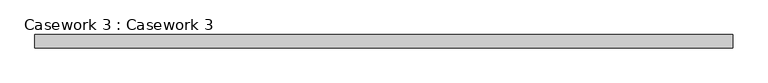
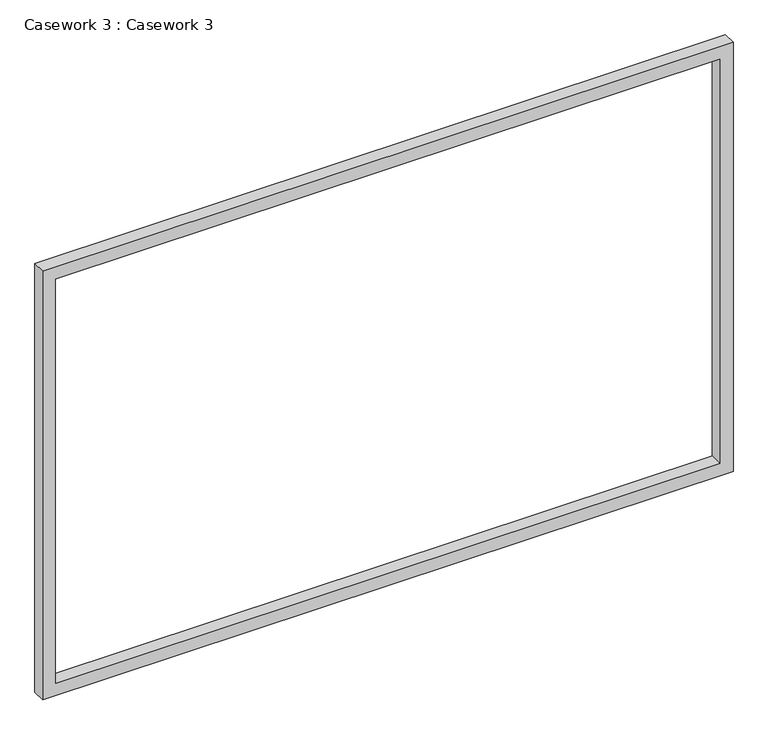
"""IFC4 building model written with IfcOpenShell, lengths in millimetres: furniture geometry, Casework 3 : Casework 3."""

from ifc_helpers import new_model, si_unit, frame, origin, place, context, project, spatial, polyline, outline, extrude, source, transform, mapped, element, save


def casework_3_casework_3_ac713c45(model_context):
    return source(origin(), model_context, "Body", "SweptSolid", [
        extrude(outline(polyline([(2895.6, -13905.4958526), (2895.6, -16572.4958526), (1143.0, -16572.4958526), (1143.0, -13905.4958526), (2895.6, -13905.4958526)]), holes=[polyline([(2844.8, -13956.2958526), (1193.8, -13956.2958526), (1193.8, -16521.6958526), (2844.8, -16521.6958526), (2844.8, -13956.2958526)])]), frame((0.0, 2993.3965218, 0.0), z_axis=(0.0, 1.0, 0.0), x_axis=(0.0, 0.0, 1.0)), (0.0, 0.0, 1.0), 50.8),
    ])


if __name__ == "__main__":
    model = new_model("IFC4")
    model_context = context("Model", 3, world=origin())
    ifc_project = project(units=[si_unit("LENGTHUNIT", "METRE", prefix="MILLI")], contexts=[model_context])
    site = spatial("IfcSite", under=ifc_project)
    building = spatial("IfcBuilding", under=site)
    placement = place(None, origin())
    casework_3_casework_3_shape = casework_3_casework_3_ac713c45(model_context)
    element("IfcFurniture", 1, ObjectType="Casework 3 : Casework 3", at=placement, inside=building, context=model_context, shape_type="MappedRepresentation", body=[
        mapped(casework_3_casework_3_shape, transform((0.0, 0.0, 0.0), x_axis=(1.0, 0.0, 0.0), y_axis=(0.0, 1.0, 0.0), z_axis=(0.0, 0.0, 1.0))),
    ])
    save(model, "model.ifc")
